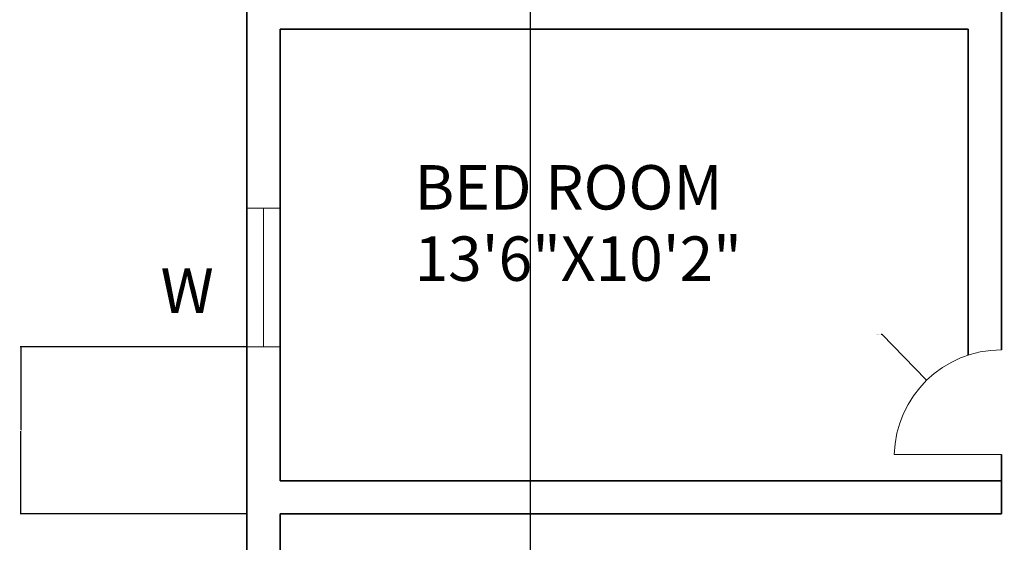
# Model space of a CAD drawing. Units: feet. Extents: x 5816 to 6644, y 25475 to 26788.
# Tile 10 of 23: x 5816 to 6082, y 26373 to 26514. Entities that reach past the tile are written whole.
import ezdxf

# ---------------------------------------------------------------- set-up
doc = ezdxf.new("R2010")
doc.units = ezdxf.units.FT
for name, color, linetype, lineweight in [('A-ANNO-DIMS', 2, 'Continuous', 13), ('A-ANNO-TEXT', 7, 'Continuous', 18), ('A-AREA-IDEN', 7, 'Continuous', 18), ('A-DOOR', 3, 'Continuous', 18), ('A-GLAZ', 4, 'Continuous', 18), ('A-WALL', 7, 'Continuous', 35)]:
    doc.layers.add(name, color=color, linetype=linetype, lineweight=lineweight)
doc.styles.get("Standard").update_dxf_attribs({"font": 'arial.ttf'})
doc.dimstyles.get("Standard").update_dxf_attribs({"dimtxt": 0.18, "dimasz": 0.18, "dimexe": 0.18, "dimexo": 0.0625, "dimgap": 0.09, "dimtad": 0, "dimtih": 1, "dimtoh": 1, "dimdec": 4, "dimzin": 0, "dimdsep": 46, "dimtxsty": 'Standard', "dimcen": 0.09, "dimadec": 0, "dimazin": 0, "dimtfac": 1, "dimtdec": 4, "dimtofl": 0, "dimtmove": 0, "dimatfit": 3, "dimfxl": 1, "dimtolj": 1, "dimtzin": 0, "dimarcsym": 0})

# ---------------------------------------------------------------- blocks, each defined once
blk = doc.blocks.new('DOOR-BEDROOM-SIDE')
blk.add_line((-28.98, 0), (0, 0))
blk.add_arc((0.03, -0.75), 29.02, 90, 178.5221)
blk = doc.blocks.new('WIN-BEDROOM-SIDE')
for p, q in [((0, 0), (9, 0)), ((4.5, 0), (4.5, -37.54)), ((0, -37.54), (9, -37.54))]:
    blk.add_line(p, q)
blk = doc.blocks.new('*D58')
at = {"layer": 'A-ANNO-DIMS', "color": 0, "lineweight": -2, "transparency": 16777216}
for p, q in [((5953.98, 26168.65), (5953.98, 26787.91)), ((5954.16, 26787.73), (6030.2, 26787.73)), ((6106.8, 26787.73), (6030.76, 26787.73)), ((6106.98, 26168.71), (6106.98, 26787.91))]:
    blk.add_line(p, q, dxfattribs=at)
at = {"layer": 'A-ANNO-DIMS', "color": 0, "transparency": 16777216}
for points in [[(5954.16, 26787.76), (5954.16, 26787.7), (5953.98, 26787.73)], [(6106.8, 26787.76), (6106.8, 26787.7), (6106.98, 26787.73)]]:
    blk.add_solid(points, dxfattribs=at)
at = {"layer": 'Defpoints', "color": 0, "transparency": 16777216}
for p in [(6106.98, 26787.73), (5953.98, 26168.58), (6106.98, 26168.65)]:
    blk.add_point(p, dxfattribs=at)
at = {"layer": 'A-ANNO-DIMS', "color": 0, "transparency": 16777216, "insert": (6030.48, 26787.73), "char_height": 0.18, "attachment_point": 5}
blk.add_mtext('\\A1;153', dxfattribs=at)
blk = doc.blocks.new('*D65')
at = {"layer": 'A-ANNO-DIMS', "color": 0, "lineweight": -2, "transparency": 16777216}
for p, q in [((5877.25, 26425.74), (5815.98, 26425.74)), ((5816.16, 26425.56), (5816.16, 26403.35)), ((5816.16, 26380.76), (5816.16, 26402.98)), ((5877.25, 26380.58), (5815.98, 26380.58))]:
    blk.add_line(p, q, dxfattribs=at)
at = {"layer": 'A-ANNO-DIMS', "color": 0, "transparency": 16777216}
for points in [[(5816.13, 26425.56), (5816.19, 26425.56), (5816.16, 26425.74)], [(5816.13, 26380.76), (5816.19, 26380.76), (5816.16, 26380.58)]]:
    blk.add_solid(points, dxfattribs=at)
at = {"layer": 'Defpoints', "color": 0, "transparency": 16777216}
for p in [(5816.16, 26425.74), (5877.31, 26425.74), (5877.31, 26380.58)]:
    blk.add_point(p, dxfattribs=at)
at = {"layer": 'A-ANNO-DIMS', "color": 0, "transparency": 16777216, "insert": (5816.16, 26403.16), "char_height": 0.18, "attachment_point": 5}
blk.add_mtext('\\A1;45.16', dxfattribs=at)
blk = doc.blocks.new('*D79')
at = {"layer": 'A-ANNO-DIMS', "color": 0, "lineweight": -2, "transparency": 16777216}
for p, q in [((6048.76, 26429.18), (6048.94, 26429.18)), ((6048.94, 26429.18), (6060.97, 26416.84)), ((6081.25, 26395.93), (6081.43, 26395.93)), ((6081.34, 26395.84), (6081.34, 26396.02))]:
    blk.add_line(p, q, dxfattribs=at)
at = {"layer": 'A-ANNO-DIMS', "color": 0, "transparency": 16777216}
blk.add_solid([(6060.99, 26416.86), (6060.94, 26416.82), (6061.09, 26416.71)], dxfattribs=at)
at = {"layer": 'Defpoints', "color": 0, "transparency": 16777216}
for p in [(6061.09, 26416.71), (6081.34, 26395.93)]:
    blk.add_point(p, dxfattribs=at)
at = {"layer": 'A-ANNO-DIMS', "color": 0, "transparency": 16777216, "insert": (6048.01, 26429.18), "char_height": 0.18, "attachment_point": 5}
blk.add_mtext('\\A1;4X R29.016', dxfattribs=at)

msp = doc.modelspace()

# ---------------------------------------------------------------- linework, layer by layer
at = {"layer": 'A-WALL'}
for p, q in [((5877.3119, 26652.5846), (5877.3119, 26253.5846)), ((6081.3119, 26530.5827), (6081.3119, 26424.9443)), ((5877.3119, 26511.5846), (5877.3119, 26253.5846)), ((5886.3119, 26511.5846), (6072.3119, 26511.5846)), ((5886.3119, 26511.5846), (5886.3119, 26389.5846)), ((6072.3119, 26511.5846), (6072.3119, 26423.5033)), ((6081.3119, 26396.677), (6081.3119, 26380.5846)), ((5886.3119, 26389.5846), (6081.3119, 26389.5846)), ((5877.3119, 26380.5846), (5877.3119, 26262.5846)), ((5886.3119, 26380.5846), (6081.3119, 26380.5846)), ((5886.3119, 26380.5846), (5886.3119, 26262.5846))]:
    msp.add_line(p, q, dxfattribs=at)

# ---------------------------------------------------------------- block references
at = {"layer": 'A-DOOR'}
msp.add_blockref('DOOR-BEDROOM-SIDE', (6081.3119, 26396.677), dxfattribs=at)
at = {"layer": 'A-GLAZ'}
msp.add_blockref('WIN-BEDROOM-SIDE', (5877.3119, 26463.2783), dxfattribs=at)

# ---------------------------------------------------------------- texts
at = {"layer": 'A-ANNO-DIMS'}
msp.add_text('13\'6"X10\'2"', height=12, dxfattribs=at).set_placement((5922.6157, 26443.5954))
at = {"layer": 'A-ANNO-TEXT'}
msp.add_text('W', height=12, dxfattribs=at).set_placement((5853.9527, 26434.9467))
at = {"layer": 'A-AREA-IDEN'}
msp.add_text('BED ROOM', height=12, dxfattribs=at).set_placement((5922.6157, 26462.8724))

# ---------------------------------------------------------------- dimensions: what is measured, and where the dimension line sits
at = {"layer": 'A-ANNO-DIMS'}
dim = msp.add_linear_dim(base=(6106.9781, 26787.7346), p1=(5953.9781, 26168.5846), p2=(6106.9781, 26168.6509), dimstyle='Standard', override={"dimdec": 0, "dimlfac": 1, "dimrnd": 0, "dimzin": 0, "dimdsep": 46, "dimlunit": 2}, dxfattribs=at)
dim.commit()
dim.dimension.update_dxf_attribs({"geometry": '*D58', "text_midpoint": (6030.4781, 26787.7346)})
dim = msp.add_radius_dim(center=(6081.3422, 26395.9287), mpoint=(6061.0913, 26416.7087), text='4X <>', dimstyle='Standard', override={"dimdec": 3, "dimlfac": 1, "dimrnd": 0, "dimzin": 0, "dimdsep": 46, "dimlunit": 2}, dxfattribs=at)
dim.commit()
dim.dimension.update_dxf_attribs({"geometry": '*D79', "text_midpoint": (6048.0141, 26429.1767), "dimtype": 164})
dim = msp.add_linear_dim(base=(5816.1619, 26425.7418), p1=(5877.3119, 26380.5846), p2=(5877.3119, 26425.7418), angle=90, dimstyle='Standard', override={"dimdec": 2, "dimlfac": 1, "dimrnd": 0, "dimzin": 0, "dimdsep": 46, "dimlunit": 2}, dxfattribs=at)
dim.commit()
dim.dimension.update_dxf_attribs({"geometry": '*D65', "text_midpoint": (5816.1619, 26403.1632)})

doc.saveas('drawing.dxf')
